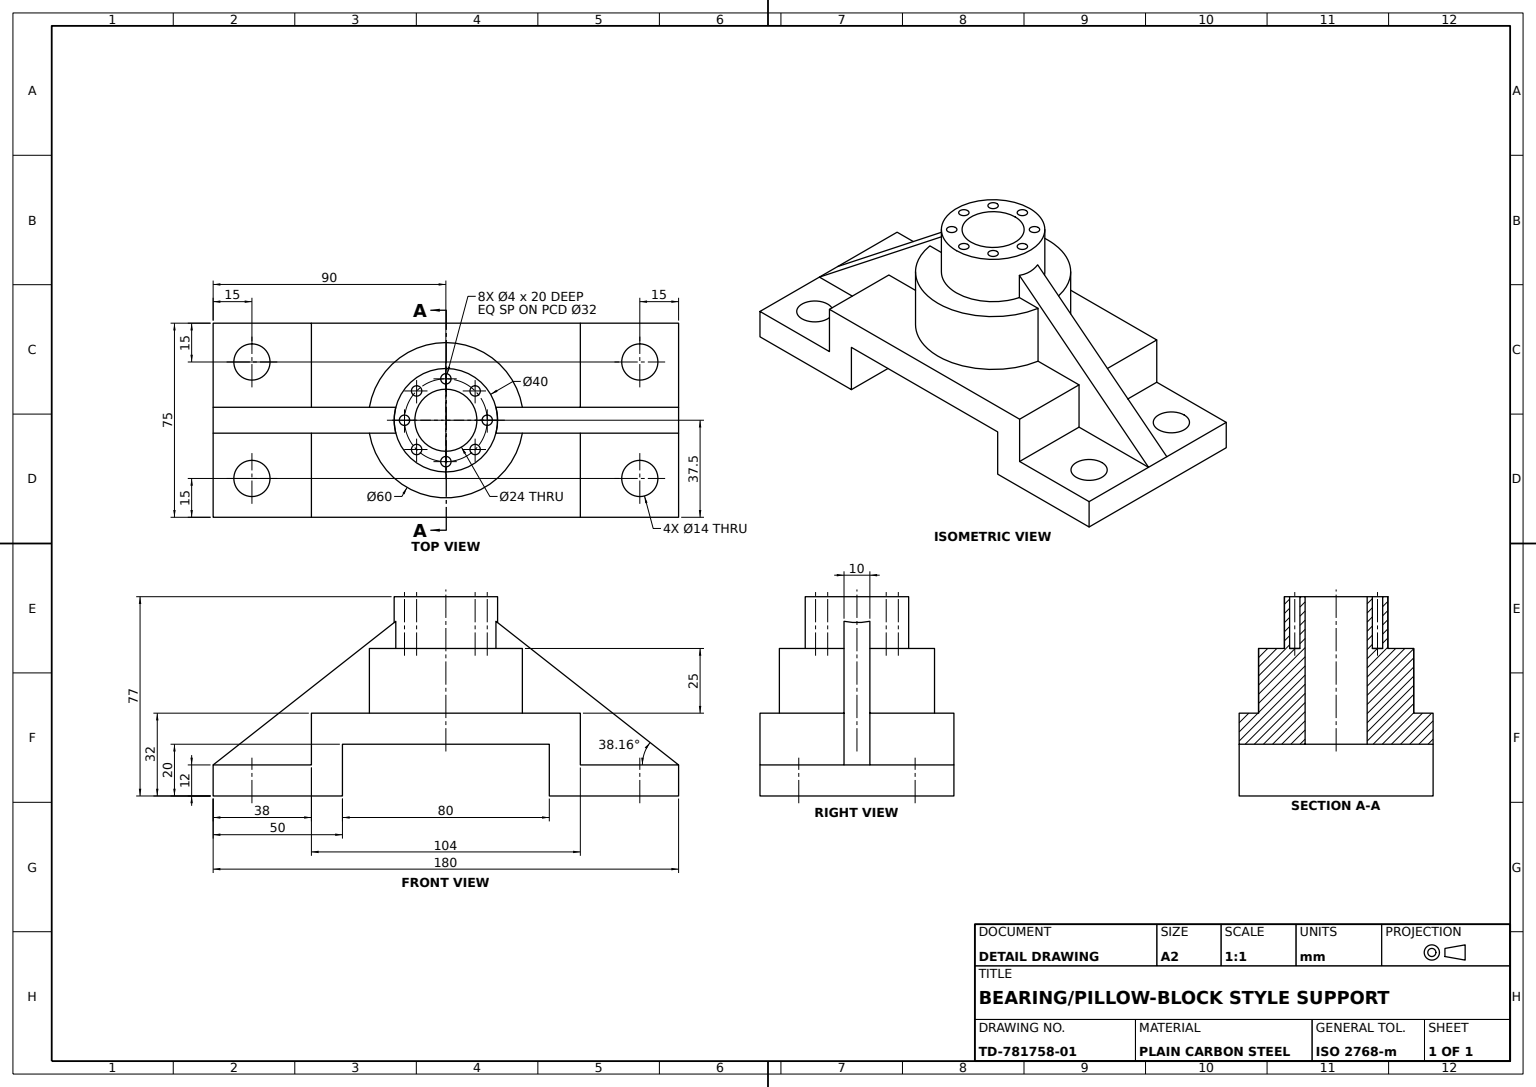
SolidWorks part; units mm, degrees
material "Plain Carbon Steel"
ref_plane "Front Plane" through (0, 0, 0) normal (0, 0, 1) x (1, 0, 0)
ref_plane "Top Plane" through (0, 0, 0) normal (0, 1, 0) x (1, 0, 0)
ref_plane "Right Plane" through (0, 0, 0) normal (1, 0, 0) x (0, 0, -1)
sketch "Base Plate Profile" plane through (0, 0, 0) normal (0, 0, 1) x (1, 0, 0)
  line L0 (0, 0) -> (50, 0)
  line L1 (50, 0) -> (50, 20)
  line L2 (50, 20) -> (130, 20)
  line L3 (130, 20) -> (130, 0)
  line L4 (130, 0) -> (180, 0)
  line L5 (180, 0) -> (180, 12)
  line L6 (180, 12) -> (142, 12)
  line L7 (142, 12) -> (142, 32)
  line L8 (142, 32) -> (38, 32)
  line L9 (38, 32) -> (38, 12)
  line L10 (38, 12) -> (0, 12)
  line L11 (0, 12) -> (0, 0)
  dimension "D1" = 50
  dimension "D2" = 20
  dimension "D3" = 80
  dimension "D4" = 12
  dimension "D5" = 38
  dimension "D6" = 50
  dimension "D7" = 104
  dimension "D8" = 20
  dimension "D9" = 12
extrude "Base Plate" add sketch "Base Plate Profile" against normal blind 75
sketch "Boss Ø60 Sketch" plane through (0, 32, 0) normal (0, 1, 0) x (1, 0, 0)
  line L0 (142, 75) -> (142, 0) construction
  line L1 (142, 0) -> (38, 0) construction
  circle A0 centre (90, 37.5) radius 30
  dimension "D1" = 60
  dimension "D2" = 52
  dimension "D3" = 37.5
extrude "Boss Ø60" add sketch "Boss Ø60 Sketch" along normal blind 25
sketch "Hub Ø40 Sketch" plane through (0, 57, 0) normal (0, 1, 0) x (1, 0, 0)
  circle A0 centre (90, 37.5) radius 20
  dimension "D1" = 40
extrude "Hub Ø40" add sketch "Hub Ø40 Sketch" along normal blind 20
sketch "Bolt Circle 8xØ4 Sketch" plane through (0, 77, 0) normal (0, 1, 0) x (1, 0, 0)
  circle A1 centre (90, 53.5) radius 2
  circle A2 centre (101.3137, 48.8137) radius 2
  circle A3 centre (106, 37.5) radius 2
  circle A4 centre (101.3137, 26.1863) radius 2
  circle A5 centre (90, 21.5) radius 2
  circle A6 centre (78.6863, 26.1863) radius 2
  circle A7 centre (74, 37.5) radius 2
  circle A8 centre (78.6863, 48.8137) radius 2
  circle A9 centre (90, 37.5) radius 20 construction
  dimension "D1" = 11.3137
  dimension "D2" = 4
  dimension "D4" = 11.3137
  dimension "D5" = 16
  dimension "D6" = 16
  dimension "D3" = 8
extrude "Bolt Circle Holes 8xØ4" cut sketch "Bolt Circle 8xØ4 Sketch" against normal blind 20
sketch "Bore Ø24 Sketch" plane through (0, 77, 0) normal (0, 1, 0) x (1, 0, 0)
  circle A0 centre (90, 37.5) radius 12
  dimension "D1" = 24
extrude "Bore Ø24" cut sketch "Bore Ø24 Sketch" against normal through all
sketch "Mounting Holes 4xØ14 Sketch" plane through (0, 12, 0) normal (0, 1, 0) x (1, 0, 0)
  line L0 (180, 0) -> (142, 0) construction
  line L1 (180, 75) -> (142, 75) construction
  line L2 (180, 75) -> (180, 0) construction
  line L3 (38, 75) -> (0, 75) construction
  line L4 (0, 75) -> (0, 0) construction
  line L5 (38, 0) -> (0, 0) construction
  circle A0 centre (165, 60) radius 7
  circle A1 centre (165, 15) radius 7
  circle A2 centre (15, 60) radius 7
  circle A3 centre (15, 15) radius 7
  dimension "D1" = 14
  dimension "D2" = 14
  dimension "D7" = 14
  dimension "D8" = 14
  dimension "D3" = 15
  dimension "D4" = 15
  dimension "D5" = 15
  dimension "D6" = 15
  dimension "D9" = 15
  dimension "D10" = 15
  dimension "D11" = 15
  dimension "D12" = 15
extrude "Mounting Holes 4xØ14" cut sketch "Mounting Holes 4xØ14 Sketch" against normal blind 20
ref_plane "Rib Mid Plane" through (0, 0, -37.5) normal (0, 0, 1) x (1, 0, 0)
sketch "Rib A Sketch" plane through (0, 0, -37.5) normal (0, 0, 1) x (1, 0, 0)
  line L0 (110, 67) -> (180, 12)
  line L1 (110, 57) -> (110, 77) construction
rib "Reinforcing Rib A" sketch "Rib A Sketch" sketch "Rib A Sketch" thickness 10 extrusion direction parallel to sketch draft on no parameters "D1"=10
sketch "Rib B Sketch" plane through (0, 0, -37.5) normal (0, 0, 1) x (1, 0, 0)
  line L0 (70, 67) -> (0, 12)
  line L1 (70, 77) -> (70, 57) construction
rib "Reinforcing Rib B" sketch "Rib B Sketch" sketch "Rib B Sketch" thickness 10 extrusion direction parallel to sketch draft on no parameters "D1"=10
